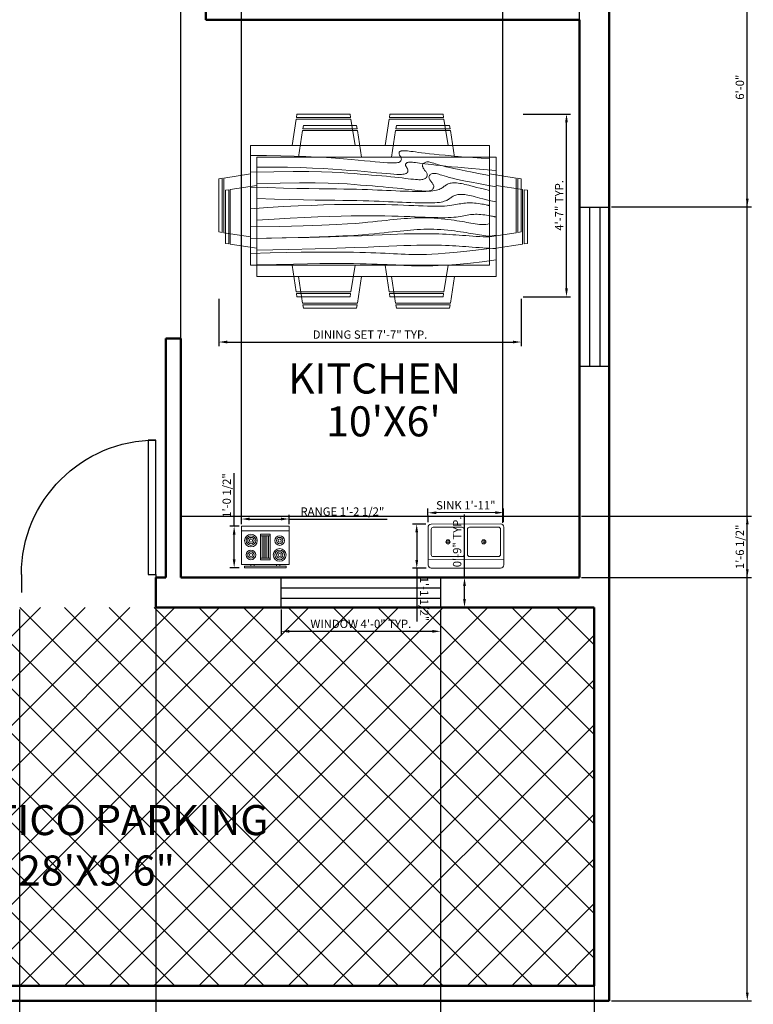
# Model space of a CAD drawing. Units: inches. Extents: x 2691 to 8091, y 3734 to 9067.
# Tile 3 of 5: x 2906 to 3127, y 3884 to 4181. Entities that reach past the tile are written whole.
import ezdxf

# ---------------------------------------------------------------- set-up
doc = ezdxf.new("R2010")
doc.units = ezdxf.units.IN
doc.layers.get('0').update_dxf_attribs({"color": 80})
for name, color, linetype, lineweight in [('A-ANNO-DIMS', 2, 'Continuous', 18), ('A-AREA-IDEN', 7, 'Continuous', 18), ('A-EQPM', 8, 'Continuous', 18), ('A-FLOR-CASE', 8, 'Continuous', 25), ('A-FLOR-FIXT', 9, 'Continuous', 18), ('A-FLOR-PATT', 252, 'Continuous', 13), ('A-FURN', 8, 'Continuous', 18), ('A-WALL', 50, 'Continuous', 50), ('doors', 10, 'Continuous', 25), ('window', 4, 'Continuous', 25)]:
    doc.layers.add(name, color=color, linetype=linetype, lineweight=lineweight)
doc.styles.get("Standard").update_dxf_attribs({"font": 'arial.ttf'})
doc.dimstyles.new('ISO-25', dxfattribs={"dimtxt": 2.5, "dimasz": 2.5, "dimexe": 1.25, "dimexo": 0.625, "dimtad": 1, "dimdec": 1, "dimlunit": 3, "dimtxsty": 'Standard', "dimcen": 2.5, "dimadec": 0, "dimazin": 0, "dimtfac": 1, "dimtdec": 1, "dimtmove": 0, "dimatfit": 3, "dimfxl": 1, "dimarcsym": 0})

# ---------------------------------------------------------------- blocks, each defined once
blk = doc.blocks.new('Dining Set - 36 x 72 in.')
for p, q in [((-22, 27.5), (-22.1562, 26.50042)), ((-22, 27.5), (-6, 27.5)), ((-5.8437, 26.49966), (-6, 27.5)), ((6, 27.5), (5.8438, 26.50042)), ((6, 27.5), (22, 27.5)), ((22.1563, 26.49966), (22, 27.5)), ((-22.2343, 26.00059), (-23.4847, 17.99762)), ((-22.2304, 26), (-5.7608, 26)), ((-5.8416, 26.5), (-22.1534, 26.5)), ((-4.5152, 17.99762), (-5.7655, 25.99926)), ((5.7657, 26.00059), (4.5153, 17.99762)), ((5.7696, 26), (22.2392, 26)), ((22.1584, 26.5), (5.8466, 26.5)), ((23.4848, 17.99762), (22.2345, 25.99926)), ((36, 18), (-36, 18)), ((-36, 18), (-36, -18)), ((36, -18), (36, 18)), ((-44.0006, 8.23428), (-35.9976, 9.48474)), ((44.0006, 8.23428), (35.9976, 9.48474)), ((-45.5, 8), (-44.5004, 8.15617)), ((-45.5, 8), (-45.5, -8)), ((-44.5, -8.15843), (-44.5, 8.15338)), ((-44, 8.23041), (-44, -8.23915)), ((44, 8.23041), (44, -8.23915)), ((44.5, -8.15843), (44.5, 8.15338)), ((45.5, 8), (44.5005, 8.15617)), ((45.5, 8), (45.5, -8)), ((-44.4997, -8.15631), (-45.5, -8)), ((-35.9976, -9.48476), (-43.9993, -8.2345)), ((35.9976, -9.48476), (43.9993, -8.2345)), ((44.4997, -8.15631), (45.5, -8)), ((-36, -18), (36, -18)), ((-22.2343, -26.0006), (-23.4847, -17.99762)), ((-4.5152, -17.99762), (-5.7655, -25.99928)), ((5.7657, -26.0006), (4.5153, -17.99762)), ((23.4848, -17.99762), (22.2345, -25.99928)), ((-22.2304, -26), (-5.7608, -26)), ((-22, -27.5), (-22.1562, -26.50044)), ((-5.8416, -26.5), (-22.1534, -26.5)), ((-5.8437, -26.49967), (-6, -27.5)), ((5.7696, -26), (22.2392, -26)), ((6, -27.5), (5.8438, -26.50044)), ((22.1584, -26.5), (5.8466, -26.5)), ((22.1563, -26.49967), (22, -27.5)), ((-22, -27.5), (-6, -27.5)), ((6, -27.5), (22, -27.5))]:
    blk.add_line(p, q)
for points in [[(-36, 15), (-31.1772, 14.97754), (-26.8079, 14.91406), (-22.8538, 14.81543), (-19.276, 14.6875), (-16.0362, 14.53613), (-13.0957, 14.36718), (-10.4159, 14.18652), (-7.9583, 14), (-5.6904, 13.81315), (-3.6035, 13.63021), (-1.6954, 13.45508), (0.0365, 13.29166), (1.5945, 13.14388), (2.9811, 13.01562), (4.1988, 12.9108), (5.25, 12.83333), (6.1393, 12.78613), (6.8802, 12.76823), (7.4883, 12.77767), (7.9792, 12.8125), (8.3685, 12.87077), (8.6719, 12.95052), (8.9049, 13.0498), (9.0833, 13.16666), (9.2205, 13.29899), (9.3216, 13.44401), (9.3895, 13.59879), (9.4271, 13.76041), (9.4373, 13.92594), (9.4232, 14.09245), (9.3875, 14.257), (9.3333, 14.41666), (9.2638, 14.56917), (9.1836, 14.71484), (9.0975, 14.85465), (9.0104, 14.98958), (8.9272, 15.1206), (8.8529, 15.2487), (8.7922, 15.37483), (8.75, 15.5), (8.7305, 15.62467), (8.7344, 15.74739), (8.7617, 15.86621), (8.8125, 15.97916), (8.8867, 16.08431), (8.9844, 16.17968), (9.1055, 16.26334), (9.25, 16.33333), (9.4189, 16.38802), (9.6172, 16.42708), (9.8506, 16.45052), (10.125, 16.45833), (10.4463, 16.45052), (10.8203, 16.42708), (11.2529, 16.38802), (11.75, 16.33333), (12.3184, 16.26318), (12.9694, 16.17838), (13.7151, 16.07991), (14.5677, 15.96875), (15.5395, 15.84586), (16.6426, 15.71224), (17.8893, 15.56884), (19.2917, 15.41666), (20.859, 15.25667), (22.5879, 15.08984), (24.4721, 14.91715), (26.5052, 14.73958), (28.6809, 14.5581), (30.9929, 14.3737), (33.4347, 14.18733), (36, 14)], [(-36, 10), (-28.9766, 10.14274), (-23.1725, 10.20442), (-18.4241, 10.19775), (-14.5677, 10.13541), (-11.4399, 10.03011), (-8.877, 9.89453), (-6.7154, 9.74137), (-4.7917, 9.58333), (-2.9698, 9.43082), (-1.2246, 9.28515), (0.4415, 9.14534), (2.026, 9.01041), (3.5266, 8.87939), (4.9408, 8.7513), (6.266, 8.62516), (7.5, 8.5), (8.6411, 8.37549), (9.6914, 8.2539), (10.6538, 8.13818), (11.5312, 8.03125), (12.3267, 7.93603), (13.043, 7.85547), (13.6831, 7.79248), (14.25, 7.75), (14.7471, 7.7303), (15.1797, 7.73307), (15.5537, 7.75732), (15.875, 7.80208), (16.1494, 7.86637), (16.3828, 7.94922), (16.5811, 8.04964), (16.75, 8.16666), (16.8944, 8.29915), (17.0143, 8.44531), (17.1089, 8.60319), (17.1771, 8.77083), (17.218, 8.94629), (17.2305, 9.1276), (17.2137, 9.31282), (17.1667, 9.5), (17.0895, 9.6875), (16.987, 9.875), (16.8649, 10.0625), (16.7292, 10.25), (16.5856, 10.4375), (16.4401, 10.625), (16.2985, 10.8125), (16.1667, 11), (16.05, 11.18733), (15.9518, 11.3737), (15.8752, 11.5581), (15.8229, 11.73958), (15.798, 11.91715), (15.8034, 12.08984), (15.842, 12.25667), (15.9167, 12.41666), (16.0295, 12.56836), (16.1784, 12.70833), (16.3605, 12.83268), (16.5729, 12.9375), (16.8127, 13.01888), (17.0768, 13.07291), (17.3625, 13.0957), (17.6667, 13.08333), (17.9894, 13.03312), (18.3418, 12.94726), (18.7382, 12.82918), (19.1927, 12.68229), (19.7195, 12.51001), (20.3327, 12.31575), (21.0465, 12.10294), (21.875, 11.875), (22.8357, 11.63354), (23.959, 11.37304), (25.2786, 11.08618), (26.8282, 10.76562), (28.6414, 10.40405), (30.752, 9.99414), (33.1936, 9.52856), (36, 9)], [(-36, 5.5), (-30.7157, 5.3348), (-26.069, 5.20963), (-21.9946, 5.11767), (-18.4271, 5.05208), (-15.3009, 5.00602), (-12.5508, 4.97265), (-10.1112, 4.94515), (-7.9167, 4.91666), (-5.909, 4.88167), (-4.0586, 4.83984), (-2.3429, 4.79215), (-0.7396, 4.73958), (0.7739, 4.6831), (2.22, 4.6237), (3.6213, 4.56233), (5, 4.5), (6.373, 4.43782), (7.7344, 4.3776), (9.0723, 4.32129), (10.375, 4.27083), (11.6309, 4.22819), (12.8281, 4.19531), (13.9551, 4.17415), (15, 4.16666), (15.954, 4.17448), (16.819, 4.19791), (17.6001, 4.23698), (18.3021, 4.29166), (18.9299, 4.36198), (19.4883, 4.44791), (19.9823, 4.54948), (20.4167, 4.66666), (20.7969, 4.79899), (21.1302, 4.94401), (21.4245, 5.09879), (21.6875, 5.26041), (21.9271, 5.42594), (22.1511, 5.59245), (22.3672, 5.757), (22.5834, 5.91666), (22.8065, 6.06868), (23.0404, 6.21093), (23.2879, 6.34147), (23.5521, 6.45833), (23.8358, 6.55957), (24.142, 6.64323), (24.4735, 6.70735), (24.8334, 6.75), (25.2235, 6.76969), (25.642, 6.76692), (26.0858, 6.74267), (26.5521, 6.69791), (27.0379, 6.63362), (27.5404, 6.55078), (28.0565, 6.45036), (28.5834, 6.33333), (29.1242, 6.19987), (29.7071, 6.04687), (30.3661, 5.87044), (31.1354, 5.66666), (32.0493, 5.43164), (33.142, 5.16146), (34.4475, 4.85221), (36, 4.5)], [(-36, -1), (-30.7915, -0.6591), (-26.0195, -0.38216), (-21.6519, -0.16284), (-17.6563, 0.00521), (-14.0005, 0.12833), (-10.6523, 0.21289), (-7.5796, 0.26522), (-4.75, 0.29166), (-2.134, 0.29793), (0.2878, 0.28711), (2.5317, 0.26163), (4.6146, 0.22396), (6.5529, 0.17651), (8.3633, 0.12174), (10.0623, 0.06209), (11.6667, 0), (13.1899, -0.06201), (14.6341, -0.1211), (15.9982, -0.17432), (17.2813, -0.21875), (18.4823, -0.25147), (19.6003, -0.26953), (20.6343, -0.27002), (21.5834, -0.25), (22.4481, -0.20768), (23.2357, -0.14584), (23.9549, -0.06836), (24.6146, 0.02083), (25.2235, 0.11784), (25.7904, 0.21875), (26.3241, 0.31966), (26.8334, 0.41666), (27.3265, 0.50618), (27.8099, 0.58593), (28.2894, 0.65397), (28.7709, 0.70833), (29.2601, 0.74707), (29.763, 0.76823), (30.2855, 0.76985), (30.8334, 0.75), (31.4088, 0.70784), (31.9994, 0.64713), (32.589, 0.57275), (33.1615, 0.48958), (33.7008, 0.4025), (34.1908, 0.3164), (34.6153, 0.23616), (34.9584, 0.16666), (35.2099, 0.11165), (35.3848, 0.07031), (35.504, 0.04069), (35.5886, 0.02083), (35.6594, 0.00879), (35.7377, 0.0026), (35.8442, 0.00032), (36, 0)], [(-36, -6.5), (-27.1843, -6.31267), (-20.084, -6.1263), (-14.469, -5.9419), (-10.1094, -5.76042), (-6.7752, -5.58285), (-4.2363, -5.41016), (-2.2629, -5.24333), (-0.625, -5.08334), (0.8708, -4.93099), (2.2715, -4.78646), (3.5872, -4.64974), (4.8281, -4.52084), (6.0046, -4.39974), (7.127, -4.28646), (8.2053, -4.18099), (9.25, -4.08334), (10.2705, -3.99382), (11.2734, -3.91407), (12.2647, -3.84603), (13.25, -3.79167), (14.2354, -3.75293), (15.2266, -3.73177), (16.2295, -3.73015), (17.25, -3.75), (18.2912, -3.79248), (19.3451, -3.85547), (20.4009, -3.93604), (21.4479, -4.03125), (22.4754, -4.13819), (23.4727, -4.25391), (24.4289, -4.37549), (25.3334, -4.5), (26.1785, -4.62492), (26.9694, -4.74935), (27.7145, -4.87281), (28.4219, -4.99479), (29.1, -5.11483), (29.7572, -5.23242), (30.4016, -5.34709), (31.0417, -5.45834), (31.6837, -5.56437), (32.3262, -5.65821), (32.9658, -5.73153), (33.599, -5.77604), (34.2224, -5.78345), (34.8327, -5.74545), (35.4264, -5.65373), (36, -5.5)], [(-36, -10), (-26.4022, -9.81299), (-18.4675, -9.62891), (-11.9839, -9.45069), (-6.7396, -9.28125), (-2.5226, -9.12354), (0.8789, -8.98047), (3.6769, -8.85498), (6.0833, -8.75), (8.2767, -8.66765), (10.3021, -8.60677), (12.1712, -8.56543), (13.8958, -8.54167), (15.4876, -8.53353), (16.9583, -8.53907), (18.3197, -8.55632), (19.5834, -8.58334), (20.7616, -8.61841), (21.8685, -8.66081), (22.9188, -8.71004), (23.9271, -8.76563), (24.9081, -8.82707), (25.8763, -8.89388), (26.8465, -8.96558), (27.8334, -9.04167), (28.8474, -9.12118), (29.8828, -9.20117), (30.93, -9.27824), (31.9792, -9.34896), (33.0205, -9.40991), (34.0443, -9.45768), (35.0407, -9.48885), (36, -9.5)], [(-36, -14.5), (-30.0881, -14.33513), (-25.0332, -14.21224), (-20.7312, -14.12647), (-17.0781, -14.07292), (-13.97, -14.04671), (-11.3027, -14.04297), (-8.9724, -14.05681), (-6.875, -14.08334), (-4.9224, -14.11833), (-3.0905, -14.16016), (-1.3709, -14.20785), (0.2448, -14.26042), (1.7647, -14.3169), (3.1973, -14.3763), (4.5507, -14.43767), (5.8333, -14.5), (7.0554, -14.5621), (8.235, -14.62175), (9.3922, -14.67652), (10.5469, -14.72396), (11.7192, -14.76164), (12.929, -14.78711), (14.1965, -14.79794), (15.5417, -14.79167), (16.9933, -14.76424), (18.6152, -14.70508), (20.4804, -14.60197), (22.6615, -14.44271), (25.2312, -14.21509), (28.2624, -13.9069), (31.8277, -13.50594), (36, -13)]]:
    blk.add_lwpolyline(points)
blk = doc.blocks.new('Sink-double - 36 in top')
for p, q in [((-18, -4), (18, -4)), ((-0.75, -18.5), (-0.75, -6.5)), ((0.75, -6.5), (0.75, -18.5))]:
    blk.add_line(p, q)
for points in [[(-16.5, 0), (16.5, 0)], [(-18, -19.5), (-18, -1.5)], [(18, -1.5), (18, -19.5)], [(-16.5, -18.5), (-16.5, -6.5)], [(-15.5, -5.5), (-1.75, -5.5)], [(1.75, -5.5), (15.5, -5.5)], [(16.5, -6.5), (16.5, -18.5)], [(16.5, -21), (-16.5, -21)], [(-1.75, -19.5), (-15.5, -19.5)], [(15.5, -19.5), (1.75, -19.5)]]:
    blk.add_lwpolyline(points)
for centre, radius in [((-8.5, -12.5), 1), ((-8.5, -12.5), 0.5), ((8.5, -12.5), 1), ((8.5, -12.5), 0.5)]:
    blk.add_circle(centre, radius)
for centre, radius, start, end in [((-16.5, -1.5), 1.5, 90, 180), ((16.5, -1.5), 1.5, 0, 90), ((-15.5, -6.5), 1, 90, 180), ((-1.75, -6.5), 1, 0, 90), ((1.75, -6.5), 1, 90, 180), ((15.5, -6.5), 1, 0, 90), ((-15.5, -18.5), 1, 180, 270), ((-1.75, -18.5), 1, 270, 0), ((1.75, -18.5), 1, 180, 270), ((15.5, -18.5), 1, 270, 0), ((-16.5, -19.5), 1.5, 180, 270), ((16.5, -19.5), 1.5, 270, 0)]:
    blk.add_arc(centre, radius, start, end)
blk = doc.blocks.new('Range-Oven - 30 in top')
for p, q in [((0, -3), (30, -3)), ((12, -6), (18, -6)), ((13, -20), (13, -6)), ((14, -6), (14, -20)), ((15, -20), (15, -6)), ((16, -6), (16, -20)), ((17, -20), (17, -6)), ((6, -24), (6, -25)), ((8, -25), (8, -24)), ((18, -20), (12, -20)), ((22, -25), (22, -24)), ((24, -24), (24, -25))]:
    blk.add_line(p, q)
for points in [[(0, -24), (0, 0), (30, 0), (30, -24)], [(12, -21), (12, -5), (18, -5), (18, -21)], [(2, -26), (2, -25), (28, -25), (28, -26)]]:
    blk.add_lwpolyline(points, close=True)
for centre, radius in [((6, -9), 4), ((6, -9), 3), ((24, -9), 3), ((6, -9), 2), ((6, -9), 1), ((24, -9), 2), ((24, -9), 1), ((6, -18), 3), ((6, -18), 2), ((6, -18), 1), ((24, -18), 4), ((24, -18), 3), ((24, -18), 2), ((24, -18), 1)]:
    blk.add_circle(centre, radius)
blk = doc.blocks.new('Dining Set - 36 x 72 in')
at = {"layer": 'window'}
for p, q in [((418.4, 887.02), (466.4, 887.02)), ((418.4, 883.92), (466.4, 883.92))]:
    blk.add_line(p, q, dxfattribs=at)
blk.add_lwpolyline([(418.4, 881.14), (418.4, 890.14), (466.4, 890.14), (466.4, 881.14)], close=True, dxfattribs=at)
blk = doc.blocks.new('*U13')
for p, q in [((0, 0), (0, -100)), ((750, 0), (750, -100))]:
    blk.add_line(p, q)
blk.add_lwpolyline([(0, 0), (0, 750), (43.75, 750), (43.75, 0)], close=True)
blk.add_arc((0, 0), 750, 0, 90)
blk = doc.blocks.new('*D21')
at = {"layer": 'A-ANNO-DIMS', "color": 0, "lineweight": -2, "transparency": 16777216}
for p, q in [((2985.17, 4003.19), (2985.17, 3995.37)), ((3033.17, 4003.19), (3033.17, 3995.37)), ((2987.67, 3996.62), (3030.67, 3996.62))]:
    blk.add_line(p, q, dxfattribs=at)
at = {"layer": 'A-ANNO-DIMS', "color": 0, "transparency": 16777216}
for points in [[(2987.67, 3997.04), (2987.67, 3996.2), (2985.17, 3996.62)], [(3030.67, 3997.04), (3030.67, 3996.2), (3033.17, 3996.62)]]:
    blk.add_solid(points, dxfattribs=at)
at = {"layer": 'Defpoints', "color": 0, "transparency": 16777216}
for p in [(2985.17, 4003.82), (3033.17, 4003.82), (3033.17, 3996.62)]:
    blk.add_point(p, dxfattribs=at)
at = {"layer": 'A-ANNO-DIMS', "color": 0, "transparency": 16777216, "insert": (3009.17, 3998.54), "char_height": 2.5, "attachment_point": 5}
blk.add_mtext('WINDOW 4\'-0" TYP.', dxfattribs=at)
blk = doc.blocks.new('*D22')
at = {"layer": 'A-ANNO-DIMS', "color": 0, "lineweight": -2, "transparency": 16777216}
for p, q in [((3040.37, 4012.82), (3040.37, 4031.81)), ((3033.8, 4012.82), (3041.62, 4012.82)), ((3040.37, 4006.32), (3040.37, 4010.32)), ((3033.8, 4003.82), (3041.62, 4003.82))]:
    blk.add_line(p, q, dxfattribs=at)
at = {"layer": 'A-ANNO-DIMS', "color": 0, "transparency": 16777216}
for points in [[(3039.96, 4010.32), (3040.79, 4010.32), (3040.37, 4012.82)], [(3039.96, 4006.32), (3040.79, 4006.32), (3040.37, 4003.82)]]:
    blk.add_solid(points, dxfattribs=at)
at = {"layer": 'Defpoints', "color": 0, "transparency": 16777216}
for p in [(3033.17, 4012.82), (3040.37, 4012.82), (3033.17, 4003.82)]:
    blk.add_point(p, dxfattribs=at)
at = {"layer": 'A-ANNO-DIMS', "color": 0, "transparency": 16777216, "insert": (3038.47, 4023.56), "char_height": 2.5, "attachment_point": 5, "rotation": 90}
blk.add_mtext('0\'-9" TYP.', dxfattribs=at)
blk = doc.blocks.new('*D33')
at = {"layer": 'A-ANNO-DIMS', "color": 0, "lineweight": -2, "transparency": 16777216}
for p, q in [((2966.43, 4096.77), (2966.43, 4082.5)), ((3057.43, 4096.77), (3057.43, 4082.5)), ((2968.93, 4083.75), (3054.93, 4083.75))]:
    blk.add_line(p, q, dxfattribs=at)
at = {"layer": 'A-ANNO-DIMS', "color": 0, "transparency": 16777216}
for points in [[(2968.93, 4084.16), (2968.93, 4083.33), (2966.43, 4083.75)], [(3054.93, 4084.16), (3054.93, 4083.33), (3057.43, 4083.75)]]:
    blk.add_solid(points, dxfattribs=at)
at = {"layer": 'Defpoints', "color": 0, "transparency": 16777216}
for p in [(2966.43, 4097.4), (3057.43, 4097.4), (3057.43, 4083.75)]:
    blk.add_point(p, dxfattribs=at)
at = {"layer": 'A-ANNO-DIMS', "color": 0, "transparency": 16777216, "insert": (3011.93, 4085.66), "char_height": 2.5, "attachment_point": 5}
blk.add_mtext('DINING SET 7\'-7" TYP.', dxfattribs=at)
blk = doc.blocks.new('*D34')
at = {"layer": 'A-ANNO-DIMS', "color": 0, "lineweight": -2, "transparency": 16777216}
for p, q in [((3058.05, 4152.4), (3072.33, 4152.4)), ((3071.08, 4099.9), (3071.08, 4149.9)), ((3058.05, 4097.4), (3072.33, 4097.4))]:
    blk.add_line(p, q, dxfattribs=at)
at = {"layer": 'A-ANNO-DIMS', "color": 0, "transparency": 16777216}
for points in [[(3070.66, 4149.9), (3071.49, 4149.9), (3071.08, 4152.4)], [(3070.66, 4099.9), (3071.49, 4099.9), (3071.08, 4097.4)]]:
    blk.add_solid(points, dxfattribs=at)
at = {"layer": 'Defpoints', "color": 0, "transparency": 16777216}
for p in [(3057.43, 4152.4), (3071.08, 4152.4), (3057.43, 4097.4)]:
    blk.add_point(p, dxfattribs=at)
at = {"layer": 'A-ANNO-DIMS', "color": 0, "transparency": 16777216, "insert": (3069.2, 4124.9), "char_height": 2.5, "attachment_point": 5, "rotation": 90}
blk.add_mtext('4\'-7" TYP.', dxfattribs=at)
blk = doc.blocks.new('*D35')
at = {"layer": 'A-ANNO-DIMS', "color": 0, "lineweight": -2, "transparency": 16777216}
for p, q in [((2973.2, 4028.91), (2973.2, 4031.69)), ((2975.7, 4030.44), (2985.12, 4030.44)), ((2987.62, 4028.91), (2987.62, 4031.69)), ((2987.62, 4030.44), (3017.1, 4030.44))]:
    blk.add_line(p, q, dxfattribs=at)
at = {"layer": 'A-ANNO-DIMS', "color": 0, "transparency": 16777216}
for points in [[(2975.7, 4030.86), (2975.7, 4030.03), (2973.2, 4030.44)], [(2985.12, 4030.86), (2985.12, 4030.03), (2987.62, 4030.44)]]:
    blk.add_solid(points, dxfattribs=at)
at = {"layer": 'Defpoints', "color": 0, "transparency": 16777216}
for p in [(2987.62, 4030.44), (2973.2, 4028.28), (2987.62, 4028.28)]:
    blk.add_point(p, dxfattribs=at)
at = {"layer": 'A-ANNO-DIMS', "color": 0, "transparency": 16777216, "insert": (3003.61, 4032.36), "char_height": 2.5, "attachment_point": 5}
blk.add_mtext('RANGE 1\'-2 1/2"', dxfattribs=at)
blk = doc.blocks.new('*D36')
at = {"layer": 'A-ANNO-DIMS', "color": 0, "lineweight": -2, "transparency": 16777216}
for p, q in [((2971.03, 4028.28), (2971.03, 4044.27)), ((2972.57, 4028.28), (2969.78, 4028.28)), ((2971.03, 4018.28), (2971.03, 4025.78)), ((2972.57, 4015.78), (2969.78, 4015.78))]:
    blk.add_line(p, q, dxfattribs=at)
at = {"layer": 'A-ANNO-DIMS', "color": 0, "transparency": 16777216}
for points in [[(2970.62, 4025.78), (2971.45, 4025.78), (2971.03, 4028.28)], [(2970.62, 4018.28), (2971.45, 4018.28), (2971.03, 4015.78)]]:
    blk.add_solid(points, dxfattribs=at)
at = {"layer": 'Defpoints', "color": 0, "transparency": 16777216}
for p in [(2971.03, 4028.28), (2973.2, 4028.28), (2973.2, 4015.78)]:
    blk.add_point(p, dxfattribs=at)
at = {"layer": 'A-ANNO-DIMS', "color": 0, "transparency": 16777216, "insert": (2969.12, 4037.52), "char_height": 2.5, "attachment_point": 5, "rotation": 90}
blk.add_mtext('1\'-0 1/2"', dxfattribs=at)
blk = doc.blocks.new('*D41')
at = {"layer": 'A-ANNO-DIMS', "color": 0, "lineweight": -2, "transparency": 16777216}
for p, q in [((3029.39, 4029.53), (3029.38, 4033.57)), ((3052.16, 4029.58), (3052.15, 4033.62)), ((3049.65, 4032.37), (3031.89, 4032.33))]:
    blk.add_line(p, q, dxfattribs=at)
at = {"layer": 'A-ANNO-DIMS', "color": 0, "transparency": 16777216}
for points in [[(3031.88, 4032.74), (3031.89, 4031.91), (3029.39, 4032.32)], [(3049.65, 4032.78), (3049.66, 4031.95), (3052.15, 4032.37)]]:
    blk.add_solid(points, dxfattribs=at)
at = {"layer": 'Defpoints', "color": 0, "transparency": 16777216}
for p in [(3029.39, 4032.32), (3029.39, 4028.91), (3052.16, 4028.96)]:
    blk.add_point(p, dxfattribs=at)
at = {"layer": 'A-ANNO-DIMS', "color": 0, "transparency": 16777216, "insert": (3040.77, 4034.26), "char_height": 2.5, "attachment_point": 5, "rotation": 0.1274}
blk.add_mtext('SINK 1\'-11"', dxfattribs=at)
blk = doc.blocks.new('*D42')
at = {"layer": 'A-ANNO-DIMS', "color": 0, "lineweight": -2, "transparency": 16777216}
for p, q in [((3028.77, 4028.91), (3024.73, 4028.9)), ((3025.98, 4026.4), (3026, 4018.12)), ((3028.8, 4015.62), (3024.76, 4015.61)), ((3026.01, 4015.62), (3026.04, 3999.63))]:
    blk.add_line(p, q, dxfattribs=at)
at = {"layer": 'A-ANNO-DIMS', "color": 0, "transparency": 16777216}
for points in [[(3026.4, 4026.4), (3025.57, 4026.4), (3025.98, 4028.9)], [(3026.42, 4018.12), (3025.58, 4018.12), (3026.01, 4015.62)]]:
    blk.add_solid(points, dxfattribs=at)
at = {"layer": 'Defpoints', "color": 0, "transparency": 16777216}
for p in [(3029.39, 4028.91), (3026.01, 4015.62), (3029.42, 4015.62)]:
    blk.add_point(p, dxfattribs=at)
at = {"layer": 'A-ANNO-DIMS', "color": 0, "transparency": 16777216, "insert": (3027.95, 4006.38), "char_height": 2.5, "attachment_point": 5, "rotation": 270.1274}
blk.add_mtext('1\'-1 1/2"', dxfattribs=at)
blk = doc.blocks.new('*D55')
at = {"layer": 'A-ANNO-DIMS', "color": 0, "lineweight": -2, "transparency": 16777216}
for p, q in [((3084.88, 4196.57), (3126.76, 4196.57)), ((3125.51, 4126.91), (3125.51, 4194.07)), ((3084.58, 4124.41), (3126.76, 4124.41))]:
    blk.add_line(p, q, dxfattribs=at)
at = {"layer": 'A-ANNO-DIMS', "color": 0, "transparency": 16777216}
for points in [[(3125.09, 4194.07), (3125.92, 4194.07), (3125.51, 4196.57)], [(3125.09, 4126.91), (3125.92, 4126.91), (3125.51, 4124.41)]]:
    blk.add_solid(points, dxfattribs=at)
at = {"layer": 'Defpoints', "color": 0, "transparency": 16777216}
for p in [(3084.26, 4196.57), (3125.51, 4196.57), (3083.96, 4124.41)]:
    blk.add_point(p, dxfattribs=at)
at = {"layer": 'A-ANNO-DIMS', "color": 0, "transparency": 16777216, "insert": (3123.6, 4160.49), "char_height": 2.5, "attachment_point": 5, "rotation": 90}
blk.add_mtext('6\'-0"', dxfattribs=at)
blk = doc.blocks.new('*D57')
at = {"layer": 'A-ANNO-DIMS', "color": 0, "lineweight": -2, "transparency": 16777216}
for p, q in [((2906.46, 4003.19), (2906.46, 3735.06)), ((2947.46, 4003.19), (2947.46, 3735.06)), ((2908.96, 3736.31), (2944.96, 3736.31))]:
    blk.add_line(p, q, dxfattribs=at)
at = {"layer": 'A-ANNO-DIMS', "color": 0, "transparency": 16777216}
for points in [[(2908.96, 3736.72), (2908.96, 3735.89), (2906.46, 3736.31)], [(2944.96, 3736.72), (2944.96, 3735.89), (2947.46, 3736.31)]]:
    blk.add_solid(points, dxfattribs=at)
at = {"layer": 'Defpoints', "color": 0, "transparency": 16777216}
for p in [(2906.46, 4003.82), (2947.46, 4003.82), (2947.46, 3736.31)]:
    blk.add_point(p, dxfattribs=at)
at = {"layer": 'A-ANNO-DIMS', "color": 0, "transparency": 16777216, "insert": (2926.96, 3738.21), "char_height": 2.5, "attachment_point": 5}
blk.add_mtext('3\'-5"', dxfattribs=at)
blk = doc.blocks.new('*D58')
at = {"layer": 'A-ANNO-DIMS', "color": 0, "lineweight": -2, "transparency": 16777216}
for p, q in [((3033.17, 4003.19), (3033.17, 3735.06)), ((3079.46, 4003.19), (3079.46, 3735.06)), ((3035.67, 3736.31), (3076.96, 3736.31))]:
    blk.add_line(p, q, dxfattribs=at)
at = {"layer": 'A-ANNO-DIMS', "color": 0, "transparency": 16777216}
for points in [[(3035.67, 3736.72), (3035.67, 3735.89), (3033.17, 3736.31)], [(3076.96, 3736.72), (3076.96, 3735.89), (3079.46, 3736.31)]]:
    blk.add_solid(points, dxfattribs=at)
at = {"layer": 'Defpoints', "color": 0, "transparency": 16777216}
for p in [(3033.17, 4003.82), (3079.46, 4003.82), (3079.46, 3736.31)]:
    blk.add_point(p, dxfattribs=at)
at = {"layer": 'A-ANNO-DIMS', "color": 0, "transparency": 16777216, "insert": (3056.32, 3738.22), "char_height": 2.5, "attachment_point": 5}
blk.add_mtext('3\'-10 1/2"', dxfattribs=at)
blk = doc.blocks.new('*D62')
at = {"layer": 'A-ANNO-DIMS', "color": 0, "lineweight": -2, "transparency": 16777216}
for p, q in [((3075.58, 4031.3), (3126.76, 4031.3)), ((3125.51, 4015.32), (3125.51, 4028.8)), ((3075.58, 4012.82), (3126.76, 4012.82))]:
    blk.add_line(p, q, dxfattribs=at)
at = {"layer": 'A-ANNO-DIMS', "color": 0, "transparency": 16777216}
for points in [[(3125.09, 4028.8), (3125.92, 4028.8), (3125.51, 4031.3)], [(3125.09, 4015.32), (3125.92, 4015.32), (3125.51, 4012.82)]]:
    blk.add_solid(points, dxfattribs=at)
at = {"layer": 'Defpoints', "color": 0, "transparency": 16777216}
for p in [(3074.96, 4031.3), (3125.51, 4031.3), (3074.96, 4012.82)]:
    blk.add_point(p, dxfattribs=at)
at = {"layer": 'A-ANNO-DIMS', "color": 0, "transparency": 16777216, "insert": (3123.59, 4022.06), "char_height": 2.5, "attachment_point": 5, "rotation": 90}
blk.add_mtext('1\'-6 1/2"', dxfattribs=at)
blk = doc.blocks.new('*D63')
at = {"layer": 'A-ANNO-DIMS', "color": 0, "lineweight": -2, "transparency": 16777216}
for p, q in [((2954.96, 4031.93), (2954.96, 4640.32)), ((2957.46, 4639.07), (2970.7, 4639.07)), ((2973.2, 4028.91), (2973.2, 4640.32))]:
    blk.add_line(p, q, dxfattribs=at)
at = {"layer": 'A-ANNO-DIMS', "color": 0, "transparency": 16777216}
for points in [[(2957.46, 4639.49), (2957.46, 4638.65), (2954.96, 4639.07)], [(2970.7, 4639.49), (2970.7, 4638.65), (2973.2, 4639.07)]]:
    blk.add_solid(points, dxfattribs=at)
at = {"layer": 'Defpoints', "color": 0, "transparency": 16777216}
for p in [(2973.2, 4639.07), (2954.96, 4031.3), (2973.2, 4028.28)]:
    blk.add_point(p, dxfattribs=at)
at = {"layer": 'A-ANNO-DIMS', "color": 0, "transparency": 16777216, "insert": (2964.08, 4640.97), "char_height": 2.5, "attachment_point": 5}
blk.add_mtext('1\'-6"', dxfattribs=at)
blk = doc.blocks.new('*D64')
at = {"layer": 'A-ANNO-DIMS', "color": 0, "lineweight": -2, "transparency": 16777216}
for p, q in [((3051.89, 4029.3), (3051.89, 4640.32)), ((3054.39, 4639.07), (3072.46, 4639.07)), ((3074.96, 4031.93), (3074.96, 4640.32))]:
    blk.add_line(p, q, dxfattribs=at)
at = {"layer": 'A-ANNO-DIMS', "color": 0, "transparency": 16777216}
for points in [[(3054.39, 4639.49), (3054.39, 4638.65), (3051.89, 4639.07)], [(3072.46, 4639.49), (3072.46, 4638.65), (3074.96, 4639.07)]]:
    blk.add_solid(points, dxfattribs=at)
at = {"layer": 'Defpoints', "color": 0, "transparency": 16777216}
for p in [(3074.96, 4639.07), (3074.96, 4031.3), (3051.89, 4028.68)]:
    blk.add_point(p, dxfattribs=at)
at = {"layer": 'A-ANNO-DIMS', "color": 0, "transparency": 16777216, "insert": (3063.42, 4640.95), "char_height": 2.5, "attachment_point": 5}
blk.add_mtext('1\'-11"', dxfattribs=at)
blk = doc.blocks.new('*D68')
at = {"layer": 'A-ANNO-DIMS', "color": 0, "lineweight": -2, "transparency": 16777216}
for p, q in [((3084.58, 4597.82), (3126.76, 4597.82)), ((3125.51, 3887.82), (3125.51, 4595.32)), ((3084.58, 3885.32), (3126.76, 3885.32))]:
    blk.add_line(p, q, dxfattribs=at)
at = {"layer": 'A-ANNO-DIMS', "color": 0, "transparency": 16777216}
for points in [[(3125.09, 4595.32), (3125.92, 4595.32), (3125.51, 4597.82)], [(3125.09, 3887.82), (3125.92, 3887.82), (3125.51, 3885.32)]]:
    blk.add_solid(points, dxfattribs=at)
at = {"layer": 'Defpoints', "color": 0, "transparency": 16777216}
for p in [(3083.96, 4597.82), (3125.51, 4597.82), (3083.96, 3885.32)]:
    blk.add_point(p, dxfattribs=at)
at = {"layer": 'A-ANNO-DIMS', "color": 0, "transparency": 16777216, "insert": (3123.59, 4241.57), "char_height": 2.5, "attachment_point": 5, "rotation": 90}
blk.add_mtext('59\'-4 1/2"', dxfattribs=at)

msp = doc.modelspace()

# ---------------------------------------------------------------- hatches: boundary and pattern name
at = {"layer": 'A-FLOR-PATT'}
h = msp.add_hatch(dxfattribs=at)
h.set_pattern_fill('ANSI37', color=256, scale=3)
h.paths.add_polyline_path([(3079.46, 4003.82), (2741.96, 4003.82), (2741.96, 3889.82), (3079.46, 3889.82)])

# ---------------------------------------------------------------- linework, layer by layer
at = {"layer": 'A-FLOR-CASE'}
msp.add_line((2954.96, 4031.3), (3074.96, 4031.3), dxfattribs=at)
at = {"layer": 'A-WALL'}
for p, q in [((3083.96, 4597.82), (3083.96, 3885.32)), ((2962.46, 4257.32), (2962.46, 4180.82)), ((2962.46, 4180.82), (3074.96, 4180.82)), ((3074.96, 4180.82), (3074.96, 4012.82)), ((2950.46, 4084.82), (2954.96, 4084.82)), ((2950.46, 4084.82), (2950.46, 4012.82)), ((2954.96, 4084.82), (2954.96, 4012.82)), ((2950.46, 4012.82), (2947.46, 4012.82)), ((2947.46, 4012.82), (2947.46, 4003.82)), ((2947.46, 4012.82), (2950.46, 4012.82)), ((2954.96, 4012.82), (3074.96, 4012.82)), ((2947.46, 4003.82), (3079.46, 4003.82)), ((3079.46, 4003.82), (3079.46, 3889.82)), ((2741.96, 3889.82), (3079.46, 3889.82)), ((2737.46, 3885.32), (3083.96, 3885.32))]:
    msp.add_line(p, q, dxfattribs=at)

# ---------------------------------------------------------------- block references
at = {"layer": 'A-EQPM', "xscale": 0.4807400298336689, "yscale": 0.4807400298336689, "zscale": 0.4807400298336689}
msp.add_blockref('Range-Oven - 30 in top', (2973.2, 4028.28), dxfattribs=at)
at = {"layer": 'A-FLOR-FIXT', "xscale": 0.632486151018198, "yscale": 0.632486151018198, "zscale": 0.632486151018198, "rotation": 180.1274480653793}
msp.add_blockref('Sink-double - 36 in top', (3040.81, 4015.65), dxfattribs=at)
at = {"layer": 'A-FURN'}
for p in [(3011.93, 4124.9), (3013.88, 4121.45)]:
    msp.add_blockref('Dining Set - 36 x 72 in.', p, dxfattribs=at)
at = {"layer": 'doors', "xscale": -0.0539913037506158, "yscale": 0.0539913037506158, "zscale": 0.0539913037506158}
msp.add_blockref('*U13', (2947.46, 4013.72), dxfattribs=at)
at = {"layer": 'window', "rotation": 90}
msp.add_blockref('Dining Set - 36 x 72 in', (3965.1, 3658), dxfattribs=at)
at = {"layer": 'window'}
msp.add_blockref('Dining Set - 36 x 72 in', (2566.77, 3122.68), dxfattribs=at)

# ---------------------------------------------------------------- texts
at = {"layer": 'A-AREA-IDEN'}
for s, height, p in [('KITCHEN', 9.054, (2987.25, 4068.23)), ("10'X6'", 9.054, (2998.72, 4055.33)), ('PORTICO PARKING', 9.0539, (2873.51, 3935.24)), ('28\'X9\'6"', 9.054, (2905.99, 3920.06))]:
    msp.add_text(s, height=height, dxfattribs=at).set_placement(p)

# ---------------------------------------------------------------- dimensions: what is measured, and where the dimension line sits
at = {"layer": 'A-ANNO-DIMS'}
for base, p1, p2, picture, middle in [((2973.2, 4639.07), (2954.96, 4031.3), (2973.2, 4028.28), '*D63', (2964.08, 4640.97)), ((3074.96, 4639.07), (3051.89, 4028.68), (3074.96, 4031.3), '*D64', (3063.42, 4640.95)), ((2947.46, 3736.31), (2906.46, 4003.82), (2947.46, 4003.82), '*D57', (2926.96, 3738.21)), ((3079.46, 3736.31), (3033.17, 4003.82), (3079.46, 4003.82), '*D58', (3056.32, 3738.22))]:
    dim = msp.add_linear_dim(base=base, p1=p1, p2=p2, dimstyle='ISO-25', override={"dimdec": 1, "dimlfac": 1, "dimrnd": 0, "dimzin": 1, "dimdsep": 46, "dimlunit": 4, "dimfrac": 2}, dxfattribs=at)
    dim.commit()
    dim.dimension.update_dxf_attribs({"geometry": picture, "text_midpoint": middle})
for base, p1, p2, angle, picture, middle in [((3125.51, 4597.82), (3083.96, 3885.32), (3083.96, 4597.82), 90, '*D68', (3123.59, 4241.57)), ((3125.51, 4196.57), (3083.96, 4124.41), (3084.26, 4196.57), 90, '*D55', (3123.6, 4160.49)), ((2971.03, 4028.28), (2973.2, 4015.78), (2973.2, 4028.28), 90, '*D36', (2969.12, 4037.52)), ((3125.51, 4031.3), (3074.96, 4012.82), (3074.96, 4031.3), 90, '*D62', (3123.59, 4022.06)), ((3026.01, 4015.62), (3029.39, 4028.91), (3029.42, 4015.62), 270.1274, '*D42', (3027.95, 4006.38))]:
    dim = msp.add_linear_dim(base=base, p1=p1, p2=p2, angle=angle, dimstyle='ISO-25', override={"dimdec": 1, "dimlfac": 1, "dimrnd": 0, "dimzin": 1, "dimdsep": 46, "dimlunit": 4, "dimfrac": 2}, dxfattribs=at)
    dim.commit()
    dim.dimension.update_dxf_attribs({"geometry": picture, "text_midpoint": middle})
for base, p1, p2, angle, text, picture, middle in [((3071.08, 4152.4), (3057.43, 4097.4), (3057.43, 4152.4), 90, '<> TYP.', '*D34', (3069.2, 4124.9)), ((3029.39, 4032.32), (3052.16, 4028.96), (3029.39, 4028.91), 180.1274, 'SINK <>', '*D41', (3040.77, 4034.26)), ((3040.37, 4012.82), (3033.17, 4003.82), (3033.17, 4012.82), 90, '<> TYP.', '*D22', (3038.47, 4023.56))]:
    dim = msp.add_linear_dim(base=base, p1=p1, p2=p2, angle=angle, text=text, dimstyle='ISO-25', override={"dimdec": 1, "dimlfac": 1, "dimrnd": 0, "dimzin": 1, "dimdsep": 46, "dimlunit": 4, "dimfrac": 2}, dxfattribs=at)
    dim.commit()
    dim.dimension.update_dxf_attribs({"geometry": picture, "text_midpoint": middle})
for base, p1, p2, text, picture, middle in [((3057.43, 4083.75), (2966.43, 4097.4), (3057.43, 4097.4), 'DINING SET <> TYP.', '*D33', (3011.93, 4085.66)), ((2987.62, 4030.44), (2973.2, 4028.28), (2987.62, 4028.28), 'RANGE <>', '*D35', (3003.61, 4032.36)), ((3033.17, 3996.62), (2985.17, 4003.82), (3033.17, 4003.82), 'WINDOW <> TYP.', '*D21', (3009.17, 3998.54))]:
    dim = msp.add_linear_dim(base=base, p1=p1, p2=p2, text=text, dimstyle='ISO-25', override={"dimdec": 1, "dimlfac": 1, "dimrnd": 0, "dimzin": 1, "dimdsep": 46, "dimlunit": 4, "dimfrac": 2}, dxfattribs=at)
    dim.commit()
    dim.dimension.update_dxf_attribs({"geometry": picture, "text_midpoint": middle})

doc.saveas('drawing.dxf')
